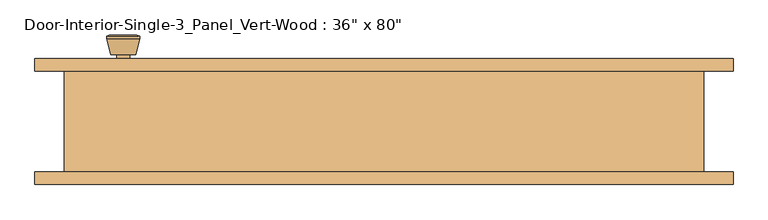
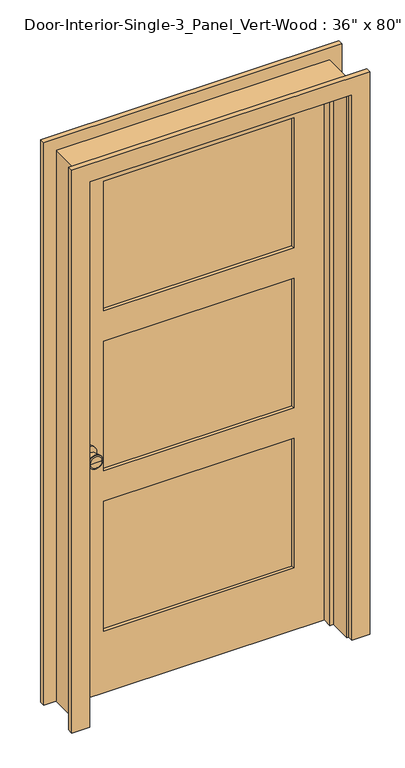
"""IFC4 building model written with IfcOpenShell, lengths in millimetres: door geometry."""

from ifc_helpers import new_model, si_unit, point, frame, frame_2d, origin, place, context, project, spatial, polyline, circle_curve, trimmed, segment, composite_curve, outline, extrude, faceted_brep, source, transform, mapped, element, save
from ifc_brep_helpers import plane_surface, cylinder_surface, revolved_surface, advanced_brep


def door_ac27962c(model_context):
    return source(origin(), model_context, "Body", "SolidModel", [
        advanced_brep(
        [(-393.7, 32.1, 914.4), (-383.7, 32.1, 914.4), (-403.7, 32.1, 914.4), (-373.2241324, -16.9, 914.4), (-393.7, -16.9, 914.4), (-414.1758676, -16.9, 914.4), (-368.7, -15.0721319, 914.4), (-418.7, -15.0721319, 914.4), (-368.7, -11.6084537, 914.4), (-418.7, -11.6084537, 914.4), (-375.063764, 13.1, 914.4), (-412.336236, 13.1, 914.4), (-383.7, 13.1, 914.4), (-403.7, 13.1, 914.4)],
        [
            (0, 1),
            (1, 2, circle_curve(frame((-393.7, 32.1, 914.4), z_axis=(0.0, 1.0, 0.0), x_axis=(-1.0, 0.0, 0.0)), 10.0)),
            (2, 0),
            (2, 1, circle_curve(frame((-393.7, 32.1, 914.4), z_axis=(0.0, 1.0, 0.0), x_axis=(-1.0, 0.0, 0.0)), 10.0)),
            (3, 4),
            (4, 5),
            (5, 3, circle_curve(frame((-393.7, -16.9, 914.4), z_axis=(0.0, -1.0, 0.0), x_axis=(-1.0, 0.0, 0.0)), 20.4758676)),
            (3, 5, circle_curve(frame((-393.7, -16.9, 914.4), z_axis=(0.0, -1.0, 0.0), x_axis=(-1.0, 0.0, 0.0)), 20.4758676)),
            (6, 3),
            (5, 7),
            (7, 6, circle_curve(frame((-393.7, -15.0721319, 914.4), z_axis=(0.0, -1.0, 0.0), x_axis=(-1.0, 0.0, 0.0)), 25.0)),
            (6, 7, circle_curve(frame((-393.7, -15.0721319, 914.4), z_axis=(0.0, -1.0, 0.0), x_axis=(-1.0, 0.0, 0.0)), 25.0)),
            (8, 6),
            (7, 9),
            (9, 8, circle_curve(frame((-393.7, -11.6084537, 914.4), z_axis=(0.0, -1.0, 0.0), x_axis=(-1.0, 0.0, 0.0)), 25.0)),
            (8, 9, circle_curve(frame((-393.7, -11.6084537, 914.4), z_axis=(0.0, -1.0, 0.0), x_axis=(-1.0, 0.0, 0.0)), 25.0)),
            (10, 8),
            (9, 11),
            (11, 10, circle_curve(frame((-393.7, 13.1, 914.4), z_axis=(0.0, -1.0, 0.0), x_axis=(-1.0, 0.0, 0.0)), 18.636236)),
            (10, 11, circle_curve(frame((-393.7, 13.1, 914.4), z_axis=(0.0, -1.0, 0.0), x_axis=(-1.0, 0.0, 0.0)), 18.636236)),
            (12, 10),
            (11, 13),
            (13, 12, circle_curve(frame((-393.7, 13.1, 914.4), z_axis=(0.0, -1.0, 0.0), x_axis=(-1.0, 0.0, 0.0)), 10.0)),
            (12, 13, circle_curve(frame((-393.7, 13.1, 914.4), z_axis=(0.0, -1.0, 0.0), x_axis=(-1.0, 0.0, 0.0)), 10.0)),
            (1, 12),
            (13, 2),
        ],
        [
            plane_surface(frame((-393.7, 32.1, 914.4), z_axis=(0.0, 1.0, 0.0), x_axis=(-1.0, 0.0, 0.0))),
            plane_surface(frame((-393.7, -16.9, 914.4), z_axis=(0.0, -1.0, 0.0), x_axis=(-1.0, 0.0, 0.0))),
            revolved_surface(polyline([(-414.1758676, -16.9, 914.4), (-418.7, -15.0721319, 914.4)]), (-393.7, 32.1, 914.4), (0.0, 1.0, 0.0)),
            cylinder_surface(frame((-393.7, 32.1, 914.4), z_axis=(0.0, 1.0, 0.0), x_axis=(-1.0, 0.0, 0.0)), 25.0),
            revolved_surface(polyline([(-418.7, -11.6084537, 914.4), (-412.336236, 13.1, 914.4)]), (-393.7, 32.1, 914.4), (0.0, 1.0, 0.0)),
            plane_surface(frame((-393.7, 13.1, 914.4), z_axis=(0.0, 1.0, 0.0), x_axis=(-1.0, 0.0, 0.0))),
            cylinder_surface(frame((-393.7, 32.1, 914.4), z_axis=(0.0, 1.0, 0.0), x_axis=(-1.0, 0.0, 0.0)), 10.0),
        ],
        [
            (0, [[1, 2, 3]]),
            (0, [[-3, 4, -1]]),
            (1, [[5, 6, 7]]),
            (1, [[-6, -5, 8]]),
            (2, [[9, -7, 10, 11]]),
            (2, [[-10, -8, -9, 12]]),
            (3, [[13, -11, 14, 15]]),
            (3, [[-14, -12, -13, 16]]),
            (4, [[17, -15, 18, 19]]),
            (4, [[-18, -16, -17, 20]]),
            (5, [[21, -19, 22, 23]]),
            (5, [[-22, -20, -21, 24]]),
            (6, [[25, -23, 26, -2]]),
            (6, [[-26, -24, -25, -4]]),
        ],
    ),
        extrude(outline(composite_curve([segment(trimmed(circle_curve(frame_2d((914.4, -393.7)), 30.0), [point((914.4, -423.7))], [point((914.4, -363.7))], False, "CARTESIAN"), True, "CONTINUOUS"), segment(trimmed(circle_curve(frame_2d((914.4, -393.7)), 30.0), [point((914.4, -363.7))], [point((914.4, -423.7))], False, "CARTESIAN"), True, "CONTINUOUS")], self_intersect=False)), frame((0.0, 32.1, 0.0), z_axis=(0.0, 1.0, 0.0), x_axis=(0.0, 0.0, 1.0)), (0.0, 0.0, 1.0), 6.0),
        advanced_brep(
        [(-393.7, 79.025, 914.4), (-403.7, 79.025, 914.4), (-383.7, 79.025, 914.4), (-373.2241324, 128.025, 914.4), (-414.1758676, 128.025, 914.4), (-393.7, 128.025, 914.4), (-368.7, 126.1971319, 914.4), (-418.7, 126.1971319, 914.4), (-368.7, 122.7334537, 914.4), (-418.7, 122.7334537, 914.4), (-375.063764, 98.025, 914.4), (-412.336236, 98.025, 914.4), (-383.7, 98.025, 914.4), (-403.7, 98.025, 914.4)],
        [
            (0, 1),
            (1, 2, circle_curve(frame((-393.7, 79.025, 914.4), z_axis=(0.0, -1.0, 0.0), x_axis=(-1.0, 0.0, 0.0)), 10.0)),
            (2, 0),
            (2, 1, circle_curve(frame((-393.7, 79.025, 914.4), z_axis=(0.0, -1.0, 0.0), x_axis=(-1.0, 0.0, 0.0)), 10.0)),
            (3, 4, circle_curve(frame((-393.7, 128.025, 914.4), z_axis=(0.0, 1.0, 0.0), x_axis=(-1.0, 0.0, 0.0)), 20.4758676)),
            (4, 5),
            (5, 3),
            (4, 3, circle_curve(frame((-393.7, 128.025, 914.4), z_axis=(0.0, 1.0, 0.0), x_axis=(-1.0, 0.0, 0.0)), 20.4758676)),
            (6, 7, circle_curve(frame((-393.7, 126.1971319, 914.4), z_axis=(0.0, 1.0, 0.0), x_axis=(-1.0, 0.0, 0.0)), 25.0)),
            (7, 4),
            (3, 6),
            (7, 6, circle_curve(frame((-393.7, 126.1971319, 914.4), z_axis=(0.0, 1.0, 0.0), x_axis=(-1.0, 0.0, 0.0)), 25.0)),
            (8, 9, circle_curve(frame((-393.7, 122.7334537, 914.4), z_axis=(0.0, 1.0, 0.0), x_axis=(-1.0, 0.0, 0.0)), 25.0)),
            (9, 7),
            (6, 8),
            (9, 8, circle_curve(frame((-393.7, 122.7334537, 914.4), z_axis=(0.0, 1.0, 0.0), x_axis=(-1.0, 0.0, 0.0)), 25.0)),
            (10, 11, circle_curve(frame((-393.7, 98.025, 914.4), z_axis=(0.0, 1.0, 0.0), x_axis=(-1.0, 0.0, 0.0)), 18.636236)),
            (11, 9),
            (8, 10),
            (11, 10, circle_curve(frame((-393.7, 98.025, 914.4), z_axis=(0.0, 1.0, 0.0), x_axis=(-1.0, 0.0, 0.0)), 18.636236)),
            (12, 13, circle_curve(frame((-393.7, 98.025, 914.4), z_axis=(0.0, 1.0, 0.0), x_axis=(-1.0, 0.0, 0.0)), 10.0)),
            (13, 11),
            (10, 12),
            (13, 12, circle_curve(frame((-393.7, 98.025, 914.4), z_axis=(0.0, 1.0, 0.0), x_axis=(-1.0, 0.0, 0.0)), 10.0)),
            (1, 13),
            (12, 2),
        ],
        [
            plane_surface(frame((-393.7, 79.025, 914.4), z_axis=(0.0, -1.0, 0.0), x_axis=(-1.0, 0.0, 0.0))),
            plane_surface(frame((-393.7, 128.025, 914.4), z_axis=(0.0, 1.0, 0.0), x_axis=(-1.0, 0.0, 0.0))),
            revolved_surface(polyline([(-414.1758676, 128.025, 914.4), (-418.7, 126.1971319, 914.4)]), (-393.7, 79.025, 914.4), (0.0, -1.0, 0.0)),
            cylinder_surface(frame((-393.7, 79.025, 914.4), z_axis=(0.0, -1.0, 0.0), x_axis=(-1.0, 0.0, 0.0)), 25.0),
            revolved_surface(polyline([(-418.7, 122.7334537, 914.4), (-412.336236, 98.025, 914.4)]), (-393.7, 79.025, 914.4), (0.0, -1.0, 0.0)),
            plane_surface(frame((-393.7, 98.025, 914.4), z_axis=(0.0, -1.0, 0.0), x_axis=(-1.0, 0.0, 0.0))),
            cylinder_surface(frame((-393.7, 79.025, 914.4), z_axis=(0.0, -1.0, 0.0), x_axis=(-1.0, 0.0, 0.0)), 10.0),
        ],
        [
            (0, [[1, 2, 3]]),
            (0, [[-3, 4, -1]]),
            (1, [[5, 6, 7]]),
            (1, [[8, -7, -6]]),
            (2, [[9, 10, -5, 11]]),
            (2, [[12, -11, -8, -10]]),
            (3, [[13, 14, -9, 15]]),
            (3, [[16, -15, -12, -14]]),
            (4, [[17, 18, -13, 19]]),
            (4, [[20, -19, -16, -18]]),
            (5, [[21, 22, -17, 23]]),
            (5, [[24, -23, -20, -22]]),
            (6, [[-2, 25, -21, 26]]),
            (6, [[-4, -26, -24, -25]]),
        ],
    ),
        extrude(outline(composite_curve([segment(trimmed(circle_curve(frame_2d((914.4, -393.7)), 30.0), [point((914.4, -423.7))], [point((914.4, -363.7))], False, "CARTESIAN"), True, "CONTINUOUS"), segment(trimmed(circle_curve(frame_2d((914.4, -393.7)), 30.0), [point((914.4, -363.7))], [point((914.4, -423.7))], False, "CARTESIAN"), True, "CONTINUOUS")], self_intersect=False)), frame((0.0, 73.025, 0.0), z_axis=(0.0, 1.0, 0.0), x_axis=(0.0, 0.0, 1.0)), (0.0, 0.0, 1.0), 6.0),
        extrude(outline(polyline([(336.55, 49.7416667), (-336.55, 49.7416667), (-336.55, 61.3833333), (336.55, 61.3833333), (336.55, 49.7416667)])), frame((0.0, 0.0, 1428.75), z_axis=(0.0, 0.0, 1.0), x_axis=(1.0, 0.0, 0.0)), (0.0, 0.0, 1.0), 484.1875),
        extrude(outline(polyline([(336.55, 49.7416667), (-336.55, 49.7416667), (-336.55, 61.3833333), (336.55, 61.3833333), (336.55, 49.7416667)])), frame((0.0, 0.0, 231.775), z_axis=(0.0, 0.0, 1.0), x_axis=(1.0, 0.0, 0.0)), (0.0, 0.0, 1.0), 484.1875),
        extrude(outline(polyline([(336.55, 49.7416667), (-336.55, 49.7416667), (-336.55, 61.3833333), (336.55, 61.3833333), (336.55, 49.7416667)])), frame((0.0, 0.0, 830.2625), z_axis=(0.0, 0.0, 1.0), x_axis=(1.0, 0.0, 0.0)), (0.0, 0.0, 1.0), 484.1875),
        extrude(outline(polyline([(2032.0, -457.2), (0.0, -457.2), (0.0, 457.2), (2032.0, 457.2), (2032.0, -457.2)]), holes=[polyline([(1912.9375, -336.55), (1912.9375, 336.55), (1428.75, 336.55), (1428.75, -336.55), (1912.9375, -336.55)]), polyline([(715.9625, -336.55), (715.9625, 336.55), (231.775, 336.55), (231.775, -336.55), (715.9625, -336.55)]), polyline([(1314.45, -336.55), (1314.45, 336.55), (830.2625, 336.55), (830.2625, -336.55), (1314.45, -336.55)])]), frame((0.0, 38.1, 0.0), z_axis=(0.0, 1.0, 0.0), x_axis=(0.0, 0.0, 1.0)), (0.0, 0.0, 1.0), 34.925),
        faceted_brep([(482.6, 73.025, 0.0), (482.6, -79.375, 0.0), (457.2, -79.375, 0.0), (457.2, 3.175, 0.0), (444.5, 3.175, 0.0), (444.5, 38.1, 0.0), (457.2, 38.1, 0.0), (457.2, 73.025, 0.0), (482.6, 73.025, 2057.4), (482.6, -79.375, 2057.4), (-482.6, -79.375, 2057.4), (-482.6, -79.375, 0.0), (-457.2, -79.375, 0.0), (-457.2, -79.375, 2032.0), (457.2, -79.375, 2032.0), (457.2, 3.175, 2032.0), (-457.2, 3.175, 2032.0), (-457.2, 3.175, 0.0), (-444.5, 3.175, 0.0), (-444.5, 3.175, 2019.3), (444.5, 3.175, 2019.3), (444.5, 38.1, 2019.3), (-444.5, 38.1, 2019.3), (-444.5, 38.1, 0.0), (-457.2, 38.1, 0.0), (-457.2, 38.1, 2032.0), (457.2, 38.1, 2032.0), (457.2, 73.025, 2032.0), (-457.2, 73.025, 2032.0), (-457.2, 73.025, 0.0), (-482.6, 73.025, 0.0), (-482.6, 73.025, 2057.4)], [[[0, 1, 2, 3, 4, 5, 6, 7]], [[1, 0, 8, 9]], [[2, 1, 9, 10, 11, 12, 13, 14]], [[3, 2, 14, 15]], [[4, 3, 15, 16, 17, 18, 19, 20]], [[5, 4, 20, 21]], [[6, 5, 21, 22, 23, 24, 25, 26]], [[7, 6, 26, 27]], [[0, 7, 27, 28, 29, 30, 31, 8]], [[9, 8, 31, 10]], [[15, 14, 13, 16]], [[21, 20, 19, 22]], [[27, 26, 25, 28]], [[30, 29, 24, 23, 18, 17, 12, 11]], [[10, 31, 30, 11]], [[16, 13, 12, 17]], [[22, 19, 18, 23]], [[28, 25, 24, 29]]]),
        extrude(outline(polyline([(0.0, 463.55), (0.0, 527.05), (2101.85, 527.05), (2101.85, -527.05), (0.0, -527.05), (0.0, -463.55), (2038.35, -463.55), (2038.35, 463.55), (0.0, 463.55)])), frame((0.0, -98.425, 0.0), z_axis=(0.0, 1.0, 0.0), x_axis=(0.0, 0.0, 1.0)), (0.0, 0.0, 1.0), 19.05),
        extrude(outline(polyline([(0.0, 463.55), (0.0, 527.05), (2101.85, 527.05), (2101.85, -527.05), (0.0, -527.05), (0.0, -463.55), (2038.35, -463.55), (2038.35, 463.55), (0.0, 463.55)])), frame((0.0, 73.025, 0.0), z_axis=(0.0, 1.0, 0.0), x_axis=(0.0, 0.0, 1.0)), (0.0, 0.0, 1.0), 19.05),
    ])


if __name__ == "__main__":
    model = new_model("IFC4")
    model_context = context("Model", 3, world=origin())
    ifc_project = project(units=[si_unit("LENGTHUNIT", "METRE", prefix="MILLI")], contexts=[model_context])
    site = spatial("IfcSite", under=ifc_project)
    building = spatial("IfcBuilding", under=site)
    placement = place(None, origin())
    door_shape = door_ac27962c(model_context)
    element("IfcDoor", 1, ObjectType="Door-Interior-Single-3_Panel_Vert-Wood : 36\" x 80\"", at=placement, inside=building, context=model_context, shape_type="MappedRepresentation", body=[
        mapped(door_shape, transform((0.0, 0.0, 0.0), x_axis=(1.0, 0.0, 0.0), y_axis=(0.0, 1.0, 0.0), z_axis=(0.0, 0.0, 1.0))),
    ])
    save(model, "model.ifc")

# Revit data of these elements
# Type "Door-Interior-Single-3_Panel_Vert-Wood : 36\" x 80\""
#   Type Mark = "10"
#   Assembly Code = "C1020300"
#   Analytic Construction = "Wooden"
#   Top Rail = 0' - 4 11/16"
#   Thickness = 0' - 1 3/8"
#   Thermal Resistance (R) = 2.5876 (h·ft²·°F)/BTU
#   Swing Angle [instance default] = 90.00°
#   Stiles = 0' - 4 3/4"
#   Rough Width = 3' - 2"
#   Rough Height = 6' - 9"
#   Intermediate Rail = 0' - 4 1/2"
#   Height = 6' - 8"
#   Width = 3' - 0"
#   Heat Transfer Coefficient (U) = 0.3865 BTU/(h·ft²·°F)
#   Bottom Rail = 0' - 9 1/8"
#   Trim Material = Cherry
#   Panel Material = Cherry
#   Frame Material = Cherry
#   Door Handle Material = Aluminum
#   Visual Light Transmittance = 0
#   Solar Heat Gain Coefficient = 0
#   Wall Closure = (empty or 0)
#   Function = (empty or 0)
# Element 1 (IfcDoor, "Door-Interior-Single-3_Panel_Vert-Wood : 36\" x 80\"")
#   Materials on its faces: "Cherry", "Aluminum"
# Materials
#   "Cherry": class "Wood", colour RGB 226 177 128, transparency 0, Description = "Prunus Serotina", Cost = 0
#   "Aluminum": class "Metal", colour RGB 247 247 247, transparency 0, Description = "Aluminum 6061", Cost = 0
